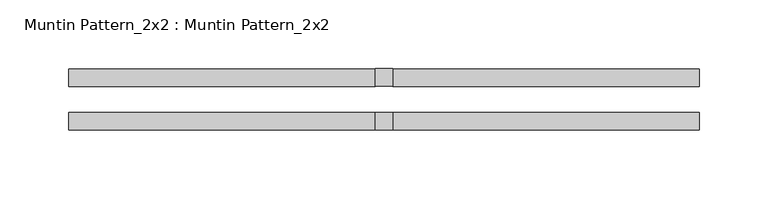
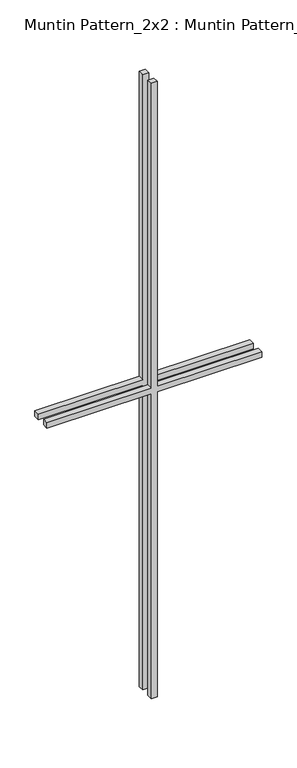
"""IFC4 building model written with IfcOpenShell, lengths in millimetres: proxy geometry, Muntin Pattern_2x2 : Muntin Pattern_2x2."""

from ifc_helpers import new_model, si_unit, frame, origin, place, context, project, spatial, polyline, outline, extrude, source, transform, mapped, element, save


def muntin_pattern_2x2_muntin_pattern_2x2_75bf01dd(model_context):
    return source(origin(), model_context, "Body", "SweptSolid", [
        extrude(outline(polyline([(698.5, -6.35), (698.5, -228.6), (685.8, -228.6), (685.8, -6.35), (0.0, -6.35), (0.0, 6.35), (685.8, 6.35), (685.8, 228.6), (698.5, 228.6), (698.5, 6.35), (1384.3, 6.35), (1384.3, -6.35), (698.5, -6.35)])), frame((0.0, 9.525, 0.0), z_axis=(0.0, 1.0, 0.0), x_axis=(0.0, 0.0, 1.0)), (0.0, 0.0, 1.0), 12.7),
        extrude(outline(polyline([(698.5, -6.35), (698.5, -228.6), (685.8, -228.6), (685.8, -6.35), (0.0, -6.35), (0.0, 6.35), (685.8, 6.35), (685.8, 228.6), (698.5, 228.6), (698.5, 6.35), (1384.3, 6.35), (1384.3, -6.35), (698.5, -6.35)])), frame((0.0, -22.225, 0.0), z_axis=(0.0, 1.0, 0.0), x_axis=(0.0, 0.0, 1.0)), (0.0, 0.0, 1.0), 12.7),
    ])


if __name__ == "__main__":
    model = new_model("IFC4")
    model_context = context("Model", 3, world=origin())
    ifc_project = project(units=[si_unit("LENGTHUNIT", "METRE", prefix="MILLI")], contexts=[model_context])
    site = spatial("IfcSite", under=ifc_project)
    building = spatial("IfcBuilding", under=site)
    placement = place(None, origin())
    muntin_pattern_2x2_muntin_pattern_2x2_shape = muntin_pattern_2x2_muntin_pattern_2x2_75bf01dd(model_context)
    element("IfcBuildingElementProxy", 1, Name="Muntin Pattern_2x2 : Muntin Pattern_2x2", ObjectType="Muntin Pattern_2x2 : Muntin Pattern_2x2", at=placement, inside=building, context=model_context, shape_type="MappedRepresentation", body=[
        mapped(muntin_pattern_2x2_muntin_pattern_2x2_shape, transform((0.0, 0.0, 0.0), x_axis=(1.0, 0.0, 0.0), y_axis=(0.0, 1.0, 0.0), z_axis=(0.0, 0.0, 1.0))),
    ])
    save(model, "model.ifc")

# Revit data of these elements
# Type "Muntin Pattern_2x2 : Muntin Pattern_2x2"
#   Width [instance default] = 4' - 0"
#   Thickness = 0' - 0 1/2"
#   Height [instance default] = 4' - 0"
#   Distance = 0' - 0 3/4"
#   Interior Material [instance default] = none
#   Exterior Material [instance default] = none
#   Default Elevation = 0
# Element 1 (IfcBuildingElementProxy, "Muntin Pattern_2x2 : Muntin Pattern_2x2")
#   Width = 1' - 6"
#   Height = 4' - 6 1/2"
#   Interior Material = Wood - Stained
#   Exterior Material = Clad - White
#   Materials on its faces: "Clad - White", "Wood - Stained"
# Materials
#   "Clad - White": class "Wood", colour RGB 30 30 30, transparency 0, Cost = 0
#   "Wood - Stained": class "Wood", colour RGB 224 178 126, transparency 0, Cost = 0
